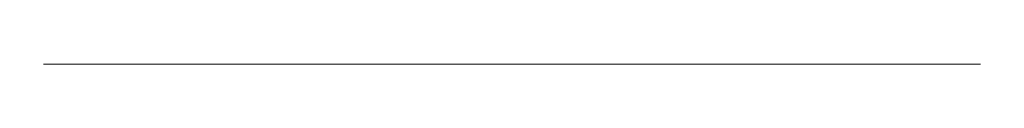
# Model space of a CAD drawing. Units: millimetres. Extents: x -35 to 77, y -482 to 0.
# Tile 2 of 2: x 49 to 77, y 0 to 0. Entities that reach past the tile are written whole.
import ezdxf

# ---------------------------------------------------------------- set-up
doc = ezdxf.new("R2010")
doc.units = ezdxf.units.MM
doc.layers.add('M-CONS', color=8, linetype='Continuous', lineweight=13)

msp = doc.modelspace()

# ---------------------------------------------------------------- linework, layer by layer
at = {"layer": 'M-CONS', "extrusion": (0, -1, 0)}
for p, q in [((60.038, 0, 183.361), (60.038, 0, 176.524)), ((60.038, 0, 176.524), (63.038, 0, 176.524)), ((63.038, 0, 176.524), (66.038, 0, 176.524)), ((66.038, 0, 176.524), (66.038, 0, 183.361))]:
    msp.add_line(p, q, dxfattribs=at)
msp.add_circle((63.038, 196.524), 8, dxfattribs=at)
msp.add_arc((63.038, 196.524), 13.5, 282.8396, 257.1604, dxfattribs=at)

doc.saveas('drawing.dxf')
